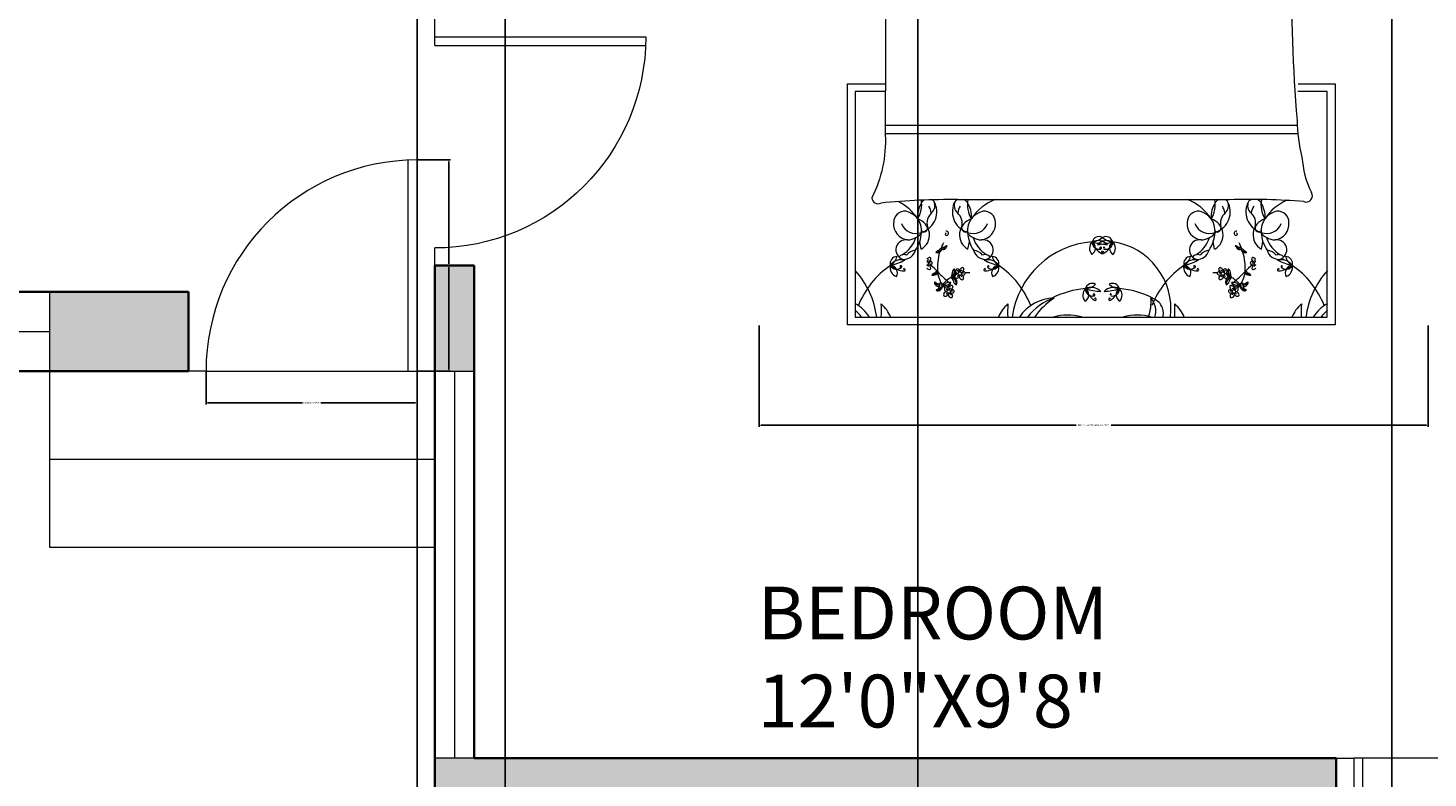
# Model space of a CAD drawing. Units: inches. Extents: x -5 to 366, y -496 to 54.
# Tile 5 of 10: x 121 to 280, y -378 to -293. Entities that reach past the tile are written whole.
import ezdxf

# ---------------------------------------------------------------- set-up
doc = ezdxf.new("R2010")
doc.units = ezdxf.units.IN
doc.header["$MEASUREMENT"] = 0
for name, color, linetype, lineweight in [('A-ANNO-DIMS', 2, 'Continuous', 18), ('A-AREA-IDEN', 7, 'Continuous', 25), ('A-DOOR', 3, 'Continuous', 18), ('A-FLOR-STRS', 7, 'Continuous', 18), ('A-FURN', 8, 'Continuous', 18), ('A-GLAZ', 4, 'Continuous', 18), ('A-WALL', 7, 'Continuous', 35), ('A-WALL-PATT', 252, 'Continuous', 13)]:
    doc.layers.add(name, color=color, linetype=linetype, lineweight=lineweight)
doc.styles.get("Standard").update_dxf_attribs({"font": 'arial.ttf'})
doc.dimstyles.get("Standard").update_dxf_attribs({"dimtxt": 0.18, "dimasz": 0.18, "dimexe": 0.18, "dimexo": 0.0625, "dimgap": 0.09, "dimtad": 0, "dimtih": 1, "dimtoh": 1, "dimdec": 0, "dimzin": 0, "dimdsep": 46, "dimlunit": 3, "dimtxsty": 'Standard', "dimcen": 0.09, "dimadec": 0, "dimazin": 0, "dimtfac": 1, "dimtdec": 0, "dimtofl": 0, "dimtmove": 0, "dimatfit": 3, "dimfxl": 1, "dimtolj": 1, "dimtzin": 0, "dimarcsym": 0})

# ---------------------------------------------------------------- blocks, each defined once
blk = doc.blocks.new('DOOR-SWING-24IN')
for p, q in [((-1, 0), (-1, 24)), ((0, 0), (0, 24))]:
    blk.add_line(p, q)
blk.add_arc((0, 0), 24, 90, 180)
blk = doc.blocks.new('BED-DOUBLE-WITH-NIGHTSTANDS')
for p, q in [((0, 64.67), (76.05, 64.67)), ((15.21, 64.67), (15.21, 43.8)), ((60.84, 63.7), (15.21, 63.7)), ((7.61, 53.37), (7.61, 63.31)), ((68.45, 53.37), (68.45, 63.31)), ((12.58, 58.34), (2.64, 58.34)), ((63.48, 58.34), (73.42, 58.34)), ((15.21, 52.66), (60.84, 52.66)), ((25.78, 50.4), (34.07, 52.66)), ((36.11, 52.66), (31.94, 46.86)), ((20.23, 48.39), (25.78, 50.4)), ((60.64, 49.5), (33.56, 49.12)), ((17.3, 46.24), (20.23, 48.39)), ((60.61, 48.72), (33, 48.33)), ((14.53, 43.01), (17.3, 46.24)), ((31.94, 46.86), (30.24, 42.39)), ((60.57, 46.32), (31.69, 46.21)), ((60.58, 45.54), (31.39, 45.42)), ((15.15, 42.39), (14.53, 43.01)), ((18.23, 42.7), (15.15, 42.39)), ((22.08, 42.39), (18.23, 42.7)), ((25.47, 41.93), (22.08, 42.39)), ((27.47, 41.01), (25.47, 41.93)), ((30.24, 42.39), (29.94, 40.39)), ((29.94, 40.39), (27.47, 41.01)), ((10.04, 27.39), (14.34, 27.39)), ((10.04, 0), (10.04, 27.39)), ((61.27, 27.39), (65.49, 27.39)), ((65.49, 27.39), (65.49, 0)), ((14.34, 26.51), (10.92, 26.51)), ((10.92, 26.51), (10.92, 0.88)), ((64.6, 26.51), (61.25, 26.51)), ((64.6, 0.88), (64.6, 26.51)), ((61.19, 22.65), (14.34, 22.65)), ((61.26, 21.7), (14.34, 21.7)), ((53.47, 14.23), (22.59, 14.23)), ((18.42, 8.59), (18.25, 9.45)), ((23.73, 8.59), (23.9, 9.45)), ((51.79, 8.59), (51.63, 9.45)), ((57.11, 8.59), (57.28, 9.45)), ((10.92, 0.88), (64.6, 0.88)), ((65.49, 0), (10.04, 0))]:
    blk.add_line(p, q)
for points in [[(15.21, 52), (0, 52), (0, 64.67)], [(60.84, 64.67), (60.84, 52), (76.05, 52), (76.05, 64.67)], [(7.61, 58.34), (8.49, 59.87)], [(68.45, 58.34), (67.56, 59.87)], [(7.61, 58.34), (8.49, 56.8)], [(68.45, 58.34), (67.56, 56.8)]]:
    blk.add_lwpolyline(points)
for points in [[(19.58, 62.78, 0.074897), (19.67, 57.81, -0.472817)], [(37.67, 57.53, 0.14099), (37.82, 62.6, 0.235245)], [(40.92, 57.53, -0.14099), (40.77, 62.6, -0.235245)], [(56.48, 62.78, -0.074897), (56.38, 57.81, 0.472817)], [(14.37, 36.04, 0.001242), (14.34, 21.61, -0.127202), (12.81, 14.42)], [(61.17, 23.25, 0.056112), (61.72, 19.07, 0.095341), (62.79, 15.03)]]:
    blk.add_lwpolyline(points, format="xyb")
for centre, radius in [((7.61, 58.34), 3.55), ((68.45, 58.34), 3.55), ((7.61, 58.34), 1.77), ((68.45, 58.34), 1.77), ((22.81, 5.83), 0.194), ((52.72, 5.83), 0.194), ((21.54, 3.79), 0.194), ((53.98, 3.79), 0.194)]:
    blk.add_circle(centre, radius)
for centre, radius, start, end in [((61.5, 786.54), 724.98, 266.68521, 267.14978), ((30, 35.26), 27.58, 82.2196, 99.497), ((35.83, 49.2), 13.55, 81.5249, 103.96), ((41.81, 58.99), 3.76, 63.3437, 106.1026), ((47.45, 49.47), 13.37, 76.3427, 101.1841), ((14.56, 786.54), 724.98, 272.85022, 273.31479), ((29.27, 55.82), 9.8, 155.1316, 191.7583), ((46.79, 55.82), 9.8, 348.2417, 24.8684), ((28.71, 54.99), 9.32, 354.0129, 15.8293), ((49.88, 54.99), 9.32, 164.1707, 185.9871), ((27.66, 70.91), 17.68, 258.0397, 289.2615), ((49.36, 62.92), 9.68, 243.8761, 286.1746), ((22.29, 63.67), 10.19, 255.1039, 281.0369), ((34.82, 67.05), 13.41, 259.8617, 283.6238), ((42.32, 57.67), 4.03, 245.0183, 288.5407), ((53.76, 63.67), 10.19, 258.9631, 284.8961), ((197.18, 43.36), 136.65, 176.1, 180.9282), ((-55.2, 41.12), 69.76, 355.8294, 1.553), ((15.83, 69.94), 28.7, 267.4519, 281.3392), ((22.69, 35.73), 6.19, 66.2616, 101.3392), ((35.22, 69.13), 29.49, 250.1194, 259.3383), ((29.76, 40.33), 0.184, 268.8623, 19.7536), ((238.78, 38.39), 178.26, 179.1145, 184.8735), ((13.51, 14.47), 0.702, 183.98, 297.3412), ((62.21, 14.65), 0.693, 246.5219, 33.8264), ((21.68, -64.93), 79.17, 89.3433, 95.6887), ((16.57, 11.64), 1.28, 84.4856, 181.0538), ((13.22, 8.88), 5.76, 33.6671, 63.2997), ((16.17, 10.69), 2.29, 355.2933, 76.921), ((20.93, 12.3), 2.93, 145.785, 184.7304), ((15.33, 13.67), 3.15, 328.8218, 9.1554), ((19.23, 13.39), 0.916, 120.0293, 142.325), ((17.77, 12.85), 2.42, 289.2822, 29.1751), ((17.4, 12.41), 2.19, 7.436, 29.9149), ((18.84, 13.57), 1.14, 311.5653, 23.8354), ((19.23, 13.39), 0.916, 44.4517, 63.558), ((24.38, 12.85), 2.42, 150.8249, 250.7178), ((23.31, 13.57), 1.14, 156.1646, 228.4347), ((22.92, 13.39), 0.916, 113.229, 135.5483), ((24.75, 12.41), 2.19, 150.0851, 172.564), ((22.92, 13.39), 0.916, 37.675, 66.7144), ((21.22, 12.3), 2.93, 355.2696, 34.215), ((26.82, 13.67), 3.15, 169.7133, 211.1782), ((25.97, 10.69), 2.29, 103.079, 184.7067), ((28.93, 8.88), 5.76, 111.4941, 146.3329), ((25.58, 11.64), 1.28, 358.9462, 95.5144), ((49.95, 11.64), 1.28, 84.4856, 181.0538), ((46.59, 8.88), 5.76, 33.6671, 68.5059), ((49.55, 10.69), 2.29, 355.2933, 76.921), ((54.31, 12.3), 2.93, 145.785, 184.7304), ((48.7, 13.67), 3.15, 328.8218, 10.2867), ((52.61, 13.39), 0.916, 113.2856, 142.325), ((51.15, 12.85), 2.42, 289.2822, 29.1751), ((50.78, 12.41), 2.19, 7.436, 29.9149), ((52.61, 13.39), 0.916, 44.4517, 66.7144), ((52.22, 13.57), 1.14, 311.5653, 23.8354), ((55.8, -59.74), 74, 85.2402, 91.8035), ((57.76, 12.85), 2.42, 150.8249, 250.7178), ((56.68, 13.57), 1.14, 156.1646, 228.4347), ((56.3, 13.39), 0.916, 106.6343, 135.5483), ((58.13, 12.41), 2.19, 150.0851, 172.564), ((56.3, 13.39), 0.916, 37.675, 72.5814), ((54.6, 12.3), 2.93, 355.2696, 34.215), ((60.2, 13.67), 3.15, 169.249, 211.1782), ((59.35, 10.69), 2.29, 103.079, 184.7067), ((62.31, 8.88), 5.76, 113.6453, 146.3329), ((58.96, 11.64), 1.28, 358.9462, 95.5144), ((17.09, 11.46), 1.82, 174.9449, 262.8857), ((17.81, 12.15), 1.76, 201.5819, 291.4221), ((17.47, 10.23), 1.89, 299.9085, 73.1337), ((18.67, 11.02), 0.472, 257.3041, 15.1471), ((20.63, 11.55), 1.56, 131.5653, 195.1471), ((21.52, 11.55), 1.56, 344.8529, 48.4347), ((24.67, 10.23), 1.89, 106.8663, 240.0915), ((23.48, 11.02), 0.472, 164.8529, 282.6959), ((24.34, 12.15), 1.76, 248.5779, 338.4181), ((25.05, 11.46), 1.82, 277.1143, 5.0551), ((50.47, 11.46), 1.82, 174.9449, 262.8857), ((51.19, 12.15), 1.76, 201.5819, 291.4221), ((50.85, 10.23), 1.89, 299.9085, 73.1337), ((52.05, 11.02), 0.472, 257.3041, 15.1471), ((54.01, 11.55), 1.56, 131.5653, 195.1471), ((54.89, 11.55), 1.56, 344.8529, 48.4347), ((58.05, 10.23), 1.89, 106.8663, 240.0915), ((56.86, 11.02), 0.472, 164.8529, 282.6959), ((57.72, 12.15), 1.76, 248.5779, 338.4181), ((58.43, 11.46), 1.82, 277.1143, 5.0551), ((16.68, 8.53), 1.14, 80.264, 250.8688), ((14.41, 11.04), 3.59, 301.2614, 341.7045), ((16.78, 11.86), 2.21, 272.3591, 324.0401), ((14.38, 10.75), 4.08, 326.2883, 356.5076), ((20.93, 12.3), 2.93, 212.7011, 216.3445), ((21.29, 10.31), 0.147, 102.7051, 280.4384), ((21.28, 10.4), 0.238, 280.4384, 100.4136), ((21.22, 12.3), 2.93, 323.6555, 327.2989), ((25.37, 11.86), 2.21, 215.9599, 267.6409), ((27.77, 10.75), 4.08, 183.4924, 213.7117), ((27.73, 11.04), 3.59, 198.2955, 238.7386), ((25.47, 8.53), 1.14, 289.1312, 99.736), ((38.64, 9.21), 0.823, 63.0274, 163.8037), ((37.8, 11.14), 1.7, 271.4585, 315.3727), ((38.49, 8.01), 1.57, 45.5411, 114.3101), ((39.57, 8.01), 1.57, 65.6899, 134.4589), ((39.42, 9.21), 0.823, 16.1963, 116.9726), ((40.26, 11.14), 1.7, 224.6273, 268.5415), ((50.06, 8.53), 1.14, 80.264, 250.8688), ((47.79, 11.04), 3.59, 301.2614, 341.7045), ((50.16, 11.86), 2.21, 272.3591, 324.0401), ((47.76, 10.75), 4.08, 326.2883, 356.5076), ((54.31, 12.3), 2.93, 212.7011, 216.3445), ((54.25, 10.4), 0.238, 79.5864, 259.5616), ((54.23, 10.31), 0.147, 259.5616, 77.2949), ((54.6, 12.3), 2.93, 323.6555, 327.2989), ((58.75, 11.86), 2.21, 215.9599, 267.6409), ((61.15, 10.75), 4.08, 183.4924, 213.7117), ((61.11, 11.04), 3.59, 198.2955, 238.7386), ((58.85, 8.53), 1.14, 289.1312, 99.736), ((16.44, 7.29), 0.7, 63.9755, 143.2681), ((16.4, 8.87), 1.43, 265.969, 344.3045), ((17.94, 6.98), 1.52, 96.1662, 141.5825), ((20.45, 8.04), 0.399, 101.3256, 154.4621), ((19.88, 9.4), 1.2, 280.2588, 300.656), ((20.15, 10.36), 2.14, 268.3264, 277.1302), ((26.56, 6.48), 6.3, 163.5842, 183.8277), ((19.62, 9.39), 1.22, 308.2101, 316.3071), ((20.37, 8.59), 0.365, 278.3432, 4.2869), ((20.17, 8.91), 0.637, 300.656, 332.6341), ((20.64, 8.49), 0.155, 55.7657, 157.4417), ((26.56, 6.48), 6.3, 153.0032, 159.8941), ((20.89, 8.63), 0.155, 84.3784, 186.0543), ((20.74, 9.25), 0.637, 269.1859, 301.164), ((20.93, 8.93), 0.365, 237.5332, 323.4768), ((20.57, 9.97), 1.22, 285.5129, 293.6099), ((21.37, 8.59), 0.399, 87.3579, 140.4944), ((20.45, 9.74), 1.2, 301.164, 321.5612), ((19.47, 9.95), 2.14, 324.6898, 333.4936), ((24.21, 6.98), 1.52, 38.4175, 83.8338), ((25.74, 8.87), 1.43, 195.6955, 274.031), ((25.71, 7.29), 0.7, 36.7319, 116.0245), ((38.62, -0.46), 9.93, 94.4623, 172.255), ((38.66, 8.7), 1.1, 137.7873, 219.1145), ((37.41, 8.74), 0.829, 298.5391, 58.3627), ((39.93, 16.07), 6.95, 252.593, 267.2582), ((38.66, 9.41), 0.812, 177.7585, 283.852), ((40.22, 10.26), 2.51, 198.9159, 238.011), ((38.14, 16.07), 6.95, 272.7418, 287.407), ((38.83, 8.73), 0.107, 283.852, 219.9245), ((38.96, 8.23), 0.123, 238.011, 71.5592), ((38.98, 8.29), 0.0599, 71.5592, 188.0167), ((39.1, 8.23), 0.123, 108.4408, 301.989), ((39.08, 8.29), 0.0599, 351.9833, 108.4408), ((39.22, 8.77), 0.0647, 320.1909, 256.0209), ((37.84, 10.26), 2.51, 301.989, 341.0841), ((39.4, 9.41), 0.812, 256.148, 2.2415), ((40.65, 8.74), 0.829, 121.6373, 241.4609), ((39.4, 8.7), 1.1, 320.8855, 42.2127), ((39.12, 1.83), 7.69, 352.8636, 81.8197), ((49.82, 7.29), 0.7, 63.9755, 143.2681), ((49.78, 8.87), 1.43, 265.969, 344.3045), ((51.32, 6.98), 1.52, 96.1662, 141.5825), ((55.08, 9.74), 1.2, 218.4388, 238.836), ((54.15, 8.59), 0.399, 39.5056, 92.6421), ((56.06, 9.95), 2.14, 206.5064, 215.3102), ((54.6, 8.93), 0.365, 216.5232, 302.4668), ((54.95, 9.97), 1.22, 246.3901, 254.4871), ((54.79, 9.25), 0.637, 238.836, 270.8141), ((48.96, 6.48), 6.3, 20.1059, 26.9968), ((54.64, 8.63), 0.155, 353.9457, 95.6216), ((54.88, 8.49), 0.155, 22.5583, 124.2343), ((55.16, 8.59), 0.365, 175.7131, 261.6568), ((55.36, 8.91), 0.637, 207.3659, 239.344), ((48.96, 6.48), 6.3, 356.1723, 16.4158), ((55.91, 9.39), 1.22, 223.6929, 231.7899), ((55.65, 9.4), 1.2, 239.344, 259.7412), ((55.37, 10.36), 2.14, 262.8698, 271.6736), ((55.07, 8.04), 0.399, 25.5379, 78.6744), ((59.12, 8.87), 1.43, 195.6955, 274.031), ((57.59, 6.98), 1.52, 38.4175, 83.8338), ((59.08, 7.29), 0.7, 36.7319, 116.0245), ((20.52, -1.44), 9.93, 124.3865, 158.5908), ((15.99, 6.52), 1.1, 167.7115, 249.0387), ((15.71, 6.95), 0.823, 92.9516, 193.728), ((14.03, 8.2), 1.7, 301.3827, 345.2969), ((16.18, 5.84), 1.57, 75.4653, 144.2343), ((13.4, 13.54), 6.95, 282.5173, 297.1824), ((14.89, 5.93), 0.829, 328.4633, 88.2869), ((16.56, 8.65), 2.51, 228.8402, 267.9352), ((15.63, 7.13), 0.812, 207.6827, 313.7762), ((16.12, 6.62), 0.107, 313.7762, 249.7183), ((16.46, 6.32), 0.0599, 101.4834, 217.9409), ((16.48, 6.26), 0.123, 267.9352, 101.4834), ((19.32, 7.28), 0.323, 101.5637, 142.6358), ((19.06, 6.98), 0.194, 273.2768, 86.7232), ((19.32, 6.63), 0.32, 217.7621, 259.0403), ((19.28, 7.17), 0.185, 91.1081, 181.8675), ((19.66, 7.05), 0.588, 203.4276, 227.6104), ((19.48, 6.8), 0.4, 80.3487, 133.6538), ((19.41, 7.13), 0.317, 229.7889, 317.6792), ((19.06, 7.54), 0.466, 288.7263, 352.5032), ((19.05, 6.46), 0.45, 355.053, 68.3618), ((19.4, 6.38), 0.634, 83.0852, 105.7171), ((19.38, 7.52), 0.15, 345.2356, 144.9248), ((19.35, 6.43), 0.149, 232.4737, 355.053), ((15.01, 1.12), 7.22, 43.1541, 52.0459), ((19.52, 7.03), 0.167, 317.6792, 80.3487), ((21.33, 6.12), 0.883, 304.5369, 16.3699), ((22.55, 5.87), 0.625, 127.3105, 187.9252), ((21.7, 5.94), 0.641, 355.0106, 41.658), ((23.08, 6.13), 0.323, 101.5637, 176.365), ((23.14, 6.36), 0.15, 345.2356, 144.9248), ((25.67, 6.26), 0.123, 78.5166, 272.0648), ((25.96, 5.84), 1.57, 35.7657, 104.5347), ((28.74, 13.54), 6.95, 242.8176, 257.4827), ((25.58, 8.65), 2.51, 272.0648, 311.1598), ((25.68, 6.32), 0.0599, 322.0591, 78.5166), ((26.52, 7.13), 0.812, 226.2238, 332.3173), ((26.04, 6.66), 0.0647, 290.2667, 226.2271), ((27.26, 5.93), 0.829, 91.7131, 211.5367), ((26.44, 6.95), 0.823, 346.272, 87.0484), ((28.12, 8.2), 1.7, 194.7031, 238.6173), ((26.16, 6.52), 1.1, 290.9613, 12.2885), ((21.63, -1.44), 9.93, 21.4092, 55.6135), ((53.9, -1.44), 9.93, 124.3865, 158.5908), ((49.36, 6.52), 1.1, 167.7115, 249.0387), ((49.09, 6.95), 0.823, 92.9516, 193.728), ((47.41, 8.2), 1.7, 301.3827, 345.2969), ((49.56, 5.84), 1.57, 75.4653, 144.2343), ((46.78, 13.54), 6.95, 282.5173, 297.1824), ((49.01, 7.13), 0.812, 207.6827, 313.7762), ((49.94, 8.65), 2.51, 228.8402, 267.9352), ((48.26, 5.93), 0.829, 328.4633, 88.2869), ((49.5, 6.62), 0.107, 313.7762, 249.7183), ((49.84, 6.32), 0.0599, 101.4834, 217.9409), ((49.86, 6.26), 0.123, 267.9352, 101.4834), ((52.39, 6.36), 0.15, 35.0752, 194.7644), ((52.45, 6.13), 0.323, 3.635, 78.4363), ((53.83, 5.94), 0.641, 138.342, 184.9894), ((54.2, 6.12), 0.883, 163.6301, 235.4631), ((52.97, 5.87), 0.625, 352.0748, 52.6895), ((60.52, 1.12), 7.22, 127.9541, 136.8459), ((56.01, 7.03), 0.167, 99.6513, 222.3208), ((56.12, 7.13), 0.317, 222.3208, 310.2111), ((56.05, 6.8), 0.4, 46.3462, 99.6513), ((56.15, 7.52), 0.15, 35.0752, 194.7644), ((56.46, 7.54), 0.466, 187.4968, 251.2737), ((56.48, 6.46), 0.45, 111.6382, 184.947), ((56.18, 6.43), 0.149, 184.947, 307.5263), ((56.12, 6.38), 0.634, 74.2829, 96.9148), ((56.25, 7.17), 0.185, 358.1325, 88.8919), ((55.86, 7.05), 0.588, 312.3896, 336.5724), ((56.2, 7.28), 0.323, 37.3642, 78.4363), ((56.21, 6.63), 0.32, 280.9597, 322.2379), ((56.47, 6.98), 0.194, 93.2768, 266.7232), ((59.05, 6.26), 0.123, 78.5166, 272.0648), ((59.34, 5.84), 1.57, 35.7657, 104.5347), ((62.12, 13.54), 6.95, 242.8176, 257.4827), ((58.96, 8.65), 2.51, 272.0648, 311.1598), ((59.06, 6.32), 0.0599, 322.0591, 78.5166), ((59.9, 7.13), 0.812, 226.2238, 332.3173), ((59.42, 6.66), 0.0647, 290.2667, 226.2271), ((60.64, 5.93), 0.829, 91.7131, 211.5367), ((61.5, 8.2), 1.7, 194.7031, 238.6173), ((59.82, 6.95), 0.823, 346.272, 87.0484), ((59.54, 6.52), 1.1, 290.9613, 12.2885), ((55.01, -1.44), 9.93, 21.4092, 55.6135), ((3.53, -0.46), 9.93, 7.745, 41.8856), ((20, 5.48), 0.399, 101.3256, 154.4621), ((19.42, 6.84), 1.2, 280.2588, 300.656), ((19.7, 7.8), 2.14, 268.3264, 277.1302), ((19.17, 6.83), 1.22, 308.2101, 316.3071), ((20.13, 4.78), 0.216, 146.8636, 236.9021), ((23.18, 9.55), 5.66, 235.1882, 238.8844), ((20.5, 5.1), 0.585, 199.4799, 267.6828), ((19.91, 6.03), 0.365, 278.3432, 4.2869), ((19.71, 6.35), 0.637, 300.656, 332.6341), ((20.19, 5.93), 0.155, 55.7657, 157.4417), ((23.43, 6.32), 3.16, 184.756, 209.2041), ((27.97, 13.04), 10.39, 222.2412, 232.1744), ((20.65, 4.61), 0.169, 311.8703, 134.2646), ((21.14, 5.38), 0.883, 247.2305, 319.0635), ((23.75, 2.13), 3.79, 120.544, 139.818), ((21.59, 4.21), 0.625, 70.0041, 130.6188), ((21.19, 4.97), 0.641, 297.7043, 344.3516), ((21.8, 5.92), 0.537, 272.8499, 356.1226), ((21.42, 5.72), 0.52, 321.7607, 7.9252), ((21.53, 4.97), 0.52, 8.7227, 54.8872), ((21.56, 4.55), 0.883, 0.278, 72.111), ((21.95, 4.88), 0.537, 20.5253, 88.5375), ((22.66, 5.14), 0.625, 188.7227, 249.3375), ((22.4, 5.47), 0.192, 148.0499, 225.6268), ((23.75, 2.13), 3.79, 113.0501, 113.8477), ((22.76, 5.25), 0.611, 104.7558, 148.0499), ((22.42, 5.69), 0.382, 247.4086, 351.4386), ((22.6, 6.1), 0.264, 126.1046, 271.4281), ((22.57, 6.17), 0.19, 353.7526, 131.7054), ((21.86, 4.83), 0.641, 334.9899, 21.6373), ((22.52, 5.67), 0.128, 262.906, 7.132), ((22.39, 5.95), 0.267, 0.0645, 61.1507), ((22.45, 6.18), 0.305, 311.8413, 355.7877), ((23.07, 5.47), 0.32, 151.2196, 259.0403), ((23.04, 6.02), 0.185, 91.1081, 181.8675), ((23.42, 5.9), 0.588, 203.4276, 227.6104), ((23.23, 5.64), 0.4, 80.3487, 133.6538), ((23.16, 5.98), 0.317, 229.7889, 317.6792), ((22.82, 6.39), 0.466, 288.7263, 352.5032), ((22.8, 5.3), 0.45, 355.053, 68.3618), ((23.16, 5.23), 0.634, 83.0852, 105.7171), ((23.1, 5.28), 0.149, 232.4737, 355.053), ((23.27, 5.87), 0.167, 317.6792, 80.3487), ((23.75, 2.13), 3.79, 87.1071, 94.7585), ((51.78, 2.13), 3.79, 85.2415, 92.8929), ((52.25, 5.87), 0.167, 99.6513, 222.3208), ((52.37, 5.98), 0.317, 222.3208, 310.2111), ((52.29, 5.64), 0.4, 46.3462, 99.6513), ((52.71, 6.39), 0.466, 187.4968, 251.2737), ((52.72, 5.3), 0.45, 111.6382, 184.947), ((52.42, 5.28), 0.149, 184.947, 307.5263), ((52.37, 5.23), 0.634, 74.2829, 96.9148), ((52.49, 6.02), 0.185, 358.1325, 88.8919), ((52.11, 5.9), 0.588, 312.3896, 336.5724), ((52.45, 5.47), 0.32, 280.9597, 28.7804), ((53.11, 5.69), 0.382, 188.5614, 292.5914), ((52.96, 6.17), 0.19, 48.2946, 186.2474), ((53.07, 6.18), 0.305, 184.2123, 228.1587), ((53.14, 5.95), 0.267, 118.8493, 179.9355), ((53, 5.67), 0.128, 172.868, 277.094), ((52.93, 6.1), 0.264, 268.5719, 53.8954), ((52.77, 5.25), 0.611, 31.9501, 75.2442), ((53.67, 4.83), 0.641, 158.3627, 205.0101), ((53.57, 4.88), 0.537, 91.4625, 159.4747), ((53.97, 4.55), 0.883, 107.889, 179.722), ((52.87, 5.14), 0.625, 290.6625, 351.2773), ((53.73, 5.92), 0.537, 183.8774, 267.1501), ((51.78, 2.13), 3.79, 66.1523, 66.9499), ((53.12, 5.47), 0.192, 314.3732, 31.9501), ((54, 4.97), 0.52, 125.1128, 171.2773), ((54.11, 5.72), 0.52, 172.0748, 218.2393), ((51.78, 2.13), 3.79, 40.182, 59.456), ((53.93, 4.21), 0.625, 49.3812, 109.9959), ((54.39, 5.38), 0.883, 220.9365, 292.7695), ((54.34, 4.97), 0.641, 195.6484, 242.2957), ((47.55, 13.04), 10.39, 307.8256, 317.7588), ((54.88, 4.61), 0.169, 45.7354, 228.1297), ((52.1, 6.32), 3.16, 330.7959, 355.244), ((55.02, 5.1), 0.585, 272.3172, 340.5201), ((55.33, 5.93), 0.155, 22.5583, 124.2343), ((55.61, 6.03), 0.365, 175.7131, 261.6568), ((55.81, 6.35), 0.637, 207.3659, 239.344), ((52.34, 9.55), 5.66, 301.1156, 304.8118), ((56.36, 6.83), 1.22, 223.6929, 231.7899), ((56.1, 6.84), 1.2, 239.344, 259.7412), ((55.39, 4.78), 0.216, 303.0979, 33.1364), ((55.82, 7.8), 2.14, 262.8698, 271.6736), ((55.53, 5.48), 0.399, 25.5379, 78.6744), ((72, -0.46), 9.93, 138.1144, 172.255), ((20.44, 4.87), 0.504, 212.8155, 277.3992), ((20.15, 4.54), 0.585, 266.9701, 338.2913), ((17.06, 8.72), 5.66, 302.6784, 306.3746), ((20.29, 4.07), 0.216, 214.3538, 304.3923), ((20.37, 4.89), 0.224, 238.8844, 314.2646), ((20.33, 4.39), 0.504, 280.3057, 17.1958), ((20.28, 4.34), 0.224, 306.3746, 21.7548), ((20.65, 4.49), 0.169, 19.3605, 201.7548), ((23.82, 3.07), 3.37, 153.7819, 158.2913), ((20.85, 5.08), 0.52, 264.4544, 310.6188), ((23.43, 6.32), 3.16, 214.0033, 222.4917), ((21.23, 4.87), 0.537, 218.3208, 298.8162), ((21.14, 3.43), 0.192, 148.0499, 225.6268), ((21.49, 3.21), 0.611, 104.7558, 148.0499), ((21.15, 3.64), 0.382, 247.4086, 351.4386), ((21.33, 4.06), 0.264, 126.1046, 271.4281), ((21.3, 4.13), 0.19, 353.7526, 131.7054), ((21.26, 3.63), 0.128, 262.906, 7.132), ((21.12, 3.91), 0.267, 0.0645, 61.1507), ((21.18, 4.13), 0.305, 311.8413, 355.7877), ((21.81, 4.09), 0.323, 101.5637, 176.365), ((21.81, 3.43), 0.32, 151.2196, 259.0403), ((21.77, 3.98), 0.185, 91.1081, 181.8675), ((22.15, 3.86), 0.588, 203.4276, 227.6104), ((21.97, 3.6), 0.4, 80.3487, 133.6538), ((21.89, 3.93), 0.317, 229.7889, 317.6792), ((21.55, 4.35), 0.466, 288.7263, 352.5032), ((21.54, 3.26), 0.45, 355.053, 68.3618), ((21.89, 3.19), 0.634, 83.0852, 105.7171), ((21.87, 4.32), 0.15, 345.2356, 144.9248), ((21.84, 3.24), 0.149, 232.4737, 355.053), ((22, 3.83), 0.167, 317.6792, 80.3487), ((37.86, -5.78), 9.93, 94.4623, 117.4146), ((37.9, 3.38), 1.1, 137.7873, 219.1145), ((36.65, 3.42), 0.829, 298.5391, 58.3627), ((37.88, 3.89), 0.823, 63.0274, 163.8037), ((37.04, 5.82), 1.7, 271.4585, 315.3727), ((37.73, 2.69), 1.57, 45.5411, 114.3101), ((39.46, 4.94), 2.51, 198.9159, 238.011), ((39.17, 10.75), 6.95, 252.593, 267.2582), ((37.9, 4.09), 0.812, 177.7585, 283.852), ((38.07, 3.41), 0.107, 283.852, 219.9245), ((40.33, 2.69), 1.57, 65.6899, 134.4589), ((38.9, 10.75), 6.95, 272.7418, 287.407), ((40.18, 3.89), 0.823, 16.1963, 116.9726), ((41.02, 5.82), 1.7, 224.6273, 268.5415), ((39.98, 3.45), 0.0647, 320.1909, 256.0209), ((38.6, 4.94), 2.51, 301.989, 341.0841), ((40.16, 4.09), 0.812, 256.148, 2.2415), ((41.41, 3.42), 0.829, 121.6373, 241.4609), ((40.16, 3.38), 1.1, 320.8855, 42.2127), ((40.2, -5.78), 9.93, 62.5854, 85.5377), ((53.52, 3.83), 0.167, 99.6513, 222.3208), ((53.63, 3.93), 0.317, 222.3208, 310.2111), ((53.56, 3.6), 0.4, 46.3462, 99.6513), ((53.66, 4.32), 0.15, 35.0752, 194.7644), ((53.97, 4.35), 0.466, 187.4968, 251.2737), ((53.99, 3.26), 0.45, 111.6382, 184.947), ((53.69, 3.24), 0.149, 184.947, 307.5263), ((53.64, 3.19), 0.634, 74.2829, 96.9148), ((53.76, 3.98), 0.185, 358.1325, 88.8919), ((53.37, 3.86), 0.588, 312.3896, 336.5724), ((53.72, 4.09), 0.323, 3.635, 78.4363), ((53.72, 3.43), 0.32, 280.9597, 28.7804), ((54.38, 3.64), 0.382, 188.5614, 292.5914), ((54.3, 4.87), 0.537, 241.1838, 321.6792), ((54.23, 4.13), 0.19, 48.2946, 186.2474), ((54.34, 4.13), 0.305, 184.2123, 228.1587), ((54.4, 3.91), 0.267, 118.8493, 179.9355), ((54.27, 3.63), 0.128, 172.868, 277.094), ((54.2, 4.06), 0.264, 268.5719, 53.8954), ((54.03, 3.21), 0.611, 31.9501, 75.2442), ((54.68, 5.08), 0.52, 229.3812, 275.5456), ((52.1, 6.32), 3.16, 317.5083, 325.9967), ((54.39, 3.43), 0.192, 314.3732, 31.9501), ((55.2, 4.39), 0.504, 162.8042, 259.6943), ((54.88, 4.49), 0.169, 338.2452, 160.6395), ((51.7, 3.07), 3.37, 21.7087, 26.2181), ((55.38, 4.54), 0.585, 201.7087, 273.0299), ((55.15, 4.89), 0.224, 225.7354, 301.1156), ((55.09, 4.87), 0.504, 262.6008, 327.1845), ((55.24, 4.34), 0.224, 158.2452, 233.6254), ((58.47, 8.72), 5.66, 233.6254, 237.3216), ((55.23, 4.07), 0.216, 235.6077, 325.6462), ((8.51, -1.79), 4.84, 33.4617, 60.1116), ((6.77, -2.69), 6.03, 36.3036, 46.4814), ((11.22, -0.67), 4.04, 22.5547, 48.9546), ((0.16, 1.5), 13.74, 357.4081, 3.6519), ((30.93, -0.67), 4.04, 131.0454, 157.4453), ((41.99, 1.5), 13.74, 176.3481, 182.5919), ((33.64, -1.79), 4.84, 91.272, 146.5383), ((35.38, -2.69), 6.03, 107.8504, 143.6964), ((38.55, -4.39), 8.97, 124.0123, 144.053), ((38.2, 2.91), 0.123, 238.011, 71.5592), ((38.22, 2.97), 0.0599, 71.5592, 188.0167), ((39.86, 2.91), 0.123, 108.4408, 301.989), ((39.84, 2.97), 0.0599, 351.9833, 108.4408), ((40.11, 2.54), 4.45, 338.117, 6.6195), ((44.19, 1.3), 1.78, 346.3898, 79.0739), ((42.85, 1.54), 2.25, 342.8609, 41.9049), ((33.54, 1.5), 13.74, 357.4081, 3.6519), ((44.6, -0.67), 4.04, 22.5547, 48.9546), ((64.31, -0.67), 4.04, 131.0454, 157.4453), ((75.37, 1.5), 13.74, 176.3481, 182.5919), ((67.02, -1.79), 4.84, 119.8884, 146.5383), ((68.76, -2.69), 6.03, 133.5186, 143.6964), ((35.08, -4.34), 5.46, 73.5431, 107.0202), ((37.25, -7.16), 8.08, 94.3787, 95.6357), ((41.5, -12.69), 14.43, 109.7217, 109.9028), ((42.98, -4.34), 5.46, 72.9798, 106.4569), ((40.82, -7.16), 8.08, 84.3643, 85.6213), ((36.56, -12.69), 14.43, 70.0972, 70.2783)]:
    blk.add_arc(centre, radius, start, end)
blk = doc.blocks.new('*D11')
at = {"layer": 'A-ANNO-DIMS', "color": 0, "lineweight": -2, "transparency": 16777216}
for p, q in [((141.43, -332.04), (141.43, -335.76)), ((165.43, -332.04), (165.43, -335.76)), ((141.61, -335.58), (152.39, -335.58)), ((165.25, -335.58), (154.48, -335.58))]:
    blk.add_line(p, q, dxfattribs=at)
at = {"layer": 'A-ANNO-DIMS', "color": 0, "transparency": 16777216}
for points in [[(141.61, -335.55), (141.61, -335.61), (141.43, -335.58)], [(165.25, -335.55), (165.25, -335.61), (165.43, -335.58)]]:
    blk.add_solid(points, dxfattribs=at)
at = {"layer": 'Defpoints', "color": 0, "transparency": 16777216}
for p in [(141.43, -331.98), (165.43, -331.98), (165.43, -335.58)]:
    blk.add_point(p, dxfattribs=at)
at = {"layer": 'A-ANNO-DIMS', "color": 0, "transparency": 16777216, "insert": (153.43, -335.58), "char_height": 0.18, "attachment_point": 5}
blk.add_mtext('\\A1;DOOR 2\'-0" TYP.', dxfattribs=at)
blk = doc.blocks.new('*D12')
at = {"layer": 'A-ANNO-DIMS', "color": 0, "lineweight": -2, "transparency": 16777216}
for p, q in [((165.5, -307.98), (169.21, -307.98)), ((169.03, -308.16), (169.03, -319.8)), ((169.03, -331.8), (169.03, -320.16)), ((165.5, -331.98), (169.21, -331.98))]:
    blk.add_line(p, q, dxfattribs=at)
at = {"layer": 'A-ANNO-DIMS', "color": 0, "transparency": 16777216}
for points in [[(169, -308.16), (169.06, -308.16), (169.03, -307.98)], [(169, -331.8), (169.06, -331.8), (169.03, -331.98)]]:
    blk.add_solid(points, dxfattribs=at)
at = {"layer": 'Defpoints', "color": 0, "transparency": 16777216}
for p in [(165.43, -307.98), (169.03, -307.98), (165.43, -331.98)]:
    blk.add_point(p, dxfattribs=at)
at = {"layer": 'A-ANNO-DIMS', "color": 0, "transparency": 16777216, "insert": (169.03, -319.98), "char_height": 0.18, "attachment_point": 5}
blk.add_mtext('\\A1;2\'-0" TYP.', dxfattribs=at)
blk = doc.blocks.new('*D15')
at = {"layer": 'A-ANNO-DIMS', "color": 0, "lineweight": -2, "transparency": 16777216}
for p, q in [((204.33, -326.78), (204.33, -338.31)), ((280.38, -326.78), (280.38, -338.31)), ((204.51, -338.13), (240.37, -338.13)), ((280.2, -338.13), (244.34, -338.13))]:
    blk.add_line(p, q, dxfattribs=at)
at = {"layer": 'A-ANNO-DIMS', "color": 0, "transparency": 16777216}
for points in [[(204.51, -338.1), (204.51, -338.16), (204.33, -338.13)], [(280.2, -338.1), (280.2, -338.16), (280.38, -338.13)]]:
    blk.add_solid(points, dxfattribs=at)
at = {"layer": 'Defpoints', "color": 0, "transparency": 16777216}
for p in [(204.33, -326.72), (280.38, -326.72), (280.38, -338.13)]:
    blk.add_point(p, dxfattribs=at)
at = {"layer": 'A-ANNO-DIMS', "color": 0, "transparency": 16777216, "insert": (242.35, -338.13), "char_height": 0.18, "attachment_point": 5}
blk.add_mtext('\\A1;BED & NIGHTSTANDS 6\'-4" TYP.', dxfattribs=at)
blk = doc.blocks.new('*D29')
at = {"layer": 'A-ANNO-DIMS', "color": 0, "lineweight": -2, "transparency": 16777216}
for p, q in [((165.43, -380.42), (165.43, 53.15)), ((165.61, 52.97), (170.03, 52.97)), ((175.25, 52.97), (170.83, 52.97)), ((175.43, -380.42), (175.43, 53.15))]:
    blk.add_line(p, q, dxfattribs=at)
at = {"layer": 'A-ANNO-DIMS', "color": 0, "transparency": 16777216}
for points in [[(165.61, 53), (165.61, 52.94), (165.43, 52.97)], [(175.25, 53), (175.25, 52.94), (175.43, 52.97)]]:
    blk.add_solid(points, dxfattribs=at)
at = {"layer": 'Defpoints', "color": 0, "transparency": 16777216}
for p in [(175.43, 52.97), (165.43, -380.48), (175.43, -380.48)]:
    blk.add_point(p, dxfattribs=at)
at = {"layer": 'A-ANNO-DIMS', "color": 0, "transparency": 16777216, "insert": (170.43, 52.97), "char_height": 0.18, "attachment_point": 5}
blk.add_mtext('\\A1;0\'-10"', dxfattribs=at)
blk = doc.blocks.new('*D32')
at = {"layer": 'A-ANNO-DIMS', "color": 0, "lineweight": -2, "transparency": 16777216}
for p, q in [((222.37, -254.15), (222.37, -495.61)), ((276.25, -254.15), (276.25, -495.61)), ((222.55, -495.43), (248.98, -495.43)), ((276.07, -495.43), (249.64, -495.43))]:
    blk.add_line(p, q, dxfattribs=at)
at = {"layer": 'A-ANNO-DIMS', "color": 0, "transparency": 16777216}
for points in [[(222.55, -495.4), (222.55, -495.46), (222.37, -495.43)], [(276.07, -495.4), (276.07, -495.46), (276.25, -495.43)]]:
    blk.add_solid(points, dxfattribs=at)
at = {"layer": 'Defpoints', "color": 0, "transparency": 16777216}
for p in [(222.37, -254.09), (276.25, -254.09), (276.25, -495.43)]:
    blk.add_point(p, dxfattribs=at)
at = {"layer": 'A-ANNO-DIMS', "color": 0, "transparency": 16777216, "insert": (249.31, -495.43), "char_height": 0.18, "attachment_point": 5}
blk.add_mtext('\\A1;4\'-6"', dxfattribs=at)

msp = doc.modelspace()

# ---------------------------------------------------------------- hatches: boundary and pattern name
at = {"layer": 'A-WALL-PATT'}
h = msp.add_hatch(color=256, dxfattribs=at)
h.dxf.hatch_style = 1
h.paths.add_polyline_path([(187.93, -13.98), (183.43, -13.98), (163.43, -13.98), (163.43, -18.48), (183.43, -18.48), (183.43, -74.48), (185.68, -74.48), (187.93, -74.48)])
h.paths.add_polyline_path([(284.93, -102.48), (215.93, -102.48), (215.93, -104.73), (215.93, -106.98), (280.43, -106.98), (284.93, -106.98)])
h.paths.add_polyline_path([(284.93, -133.23), (280.43, -133.23), (280.43, -154.98), (220.43, -154.98), (220.43, -134.98), (215.93, -134.98), (215.93, -159.48), (284.93, -159.48)])
h.paths.add_polyline_path([(139.43, -322.98), (123.64, -322.98), (123.64, -331.98), (139.43, -331.98)])
h.paths.add_polyline_path([(171.93, -319.98), (167.43, -319.98), (167.43, -331.98), (171.93, -331.98)])
h.paths.add_polyline_path([(269.93, -375.98), (171.93, -375.98), (167.43, -375.98), (167.43, -380.48), (171.93, -380.48), (265.43, -380.48), (265.43, -452.48), (171.93, -452.48), (167.43, -452.48), (167.43, -456.98), (281.67, -456.98), (281.67, -452.48), (269.93, -452.48), (269.93, -380.48)])

# ---------------------------------------------------------------- linework, layer by layer
at = {"layer": 'A-DOOR'}
for p, q in [((167.43, -294.98), (167.43, -291.98)), ((167.43, -319.98), (167.43, -317.98)), ((141.43, -331.98), (139.43, -331.98)), ((141.43, -331.98), (165.43, -331.98)), ((167.43, -331.98), (165.43, -331.98)), ((269.93, -375.98), (271.93, -375.98)), ((295.93, -375.98), (271.93, -375.98))]:
    msp.add_line(p, q, dxfattribs=at)
at = {"layer": 'A-FLOR-STRS'}
for p, q in [((123.64, -331.98), (123.64, -341.98)), ((123.64, -341.98), (123.64, -351.98)), ((123.64, -341.98), (167.43, -341.98)), ((123.64, -351.98), (167.43, -351.98))]:
    msp.add_line(p, q, dxfattribs=at)
at = {"layer": 'A-GLAZ'}
for p, q in [((123.64, -322.98), (123.64, -331.98)), ((30.93, -327.48), (123.64, -327.48)), ((167.43, -331.98), (171.93, -331.98)), ((169.68, -331.98), (169.68, -375.98)), ((171.93, -375.98), (167.43, -375.98))]:
    msp.add_line(p, q, dxfattribs=at)
at = {"layer": 'A-WALL'}
for p, q in [((171.93, -319.98), (167.43, -319.98)), ((167.43, -319.98), (167.43, -380.48)), ((171.93, -319.98), (171.93, -375.98)), ((30.93, -322.98), (139.43, -322.98)), ((139.43, -331.98), (139.43, -322.98)), ((26.43, -331.98), (139.43, -331.98)), ((171.93, -375.98), (269.93, -375.98)), ((269.93, -380.48), (269.93, -375.98))]:
    msp.add_line(p, q, dxfattribs=at)

# ---------------------------------------------------------------- block references
at = {"layer": 'A-DOOR', "extrusion": (0, 0, -1), "zscale": -1, "rotation": 90.00000000000007}
msp.add_blockref('DOOR-SWING-24IN', (-167.43, -293.98), dxfattribs=at)
at = {"layer": 'A-DOOR'}
msp.add_blockref('DOOR-SWING-24IN', (165.43, -331.98), dxfattribs=at)
at = {"layer": 'A-DOOR', "rotation": 180}
msp.add_blockref('DOOR-SWING-24IN', (271.93, -375.98), dxfattribs=at)
at = {"layer": 'A-FURN'}
msp.add_blockref('BED-DOUBLE-WITH-NIGHTSTANDS', (204.33, -326.72), dxfattribs=at)

# ---------------------------------------------------------------- texts
at = {"layer": 'A-AREA-IDEN', "insert": (204.16, -356.48), "char_height": 6, "attachment_point": 1}
msp.add_mtext('BEDROOM\\P12\'0"X9\'8"', dxfattribs=at)

# ---------------------------------------------------------------- dimensions: what is measured, and where the dimension line sits
at = {"layer": 'A-ANNO-DIMS'}
for base, p1, p2, picture, middle in [((175.43, 52.97), (165.43, -380.48), (175.43, -380.48), '*D29', (170.43, 52.97)), ((276.25, -495.43), (222.37, -254.09), (276.25, -254.09), '*D32', (249.31, -495.43))]:
    dim = msp.add_linear_dim(base=base, p1=p1, p2=p2, dimstyle='Standard', override={"dimdec": 1, "dimlfac": 1, "dimrnd": 0, "dimzin": 1, "dimdsep": 46, "dimlunit": 4, "dimfrac": 2}, dxfattribs=at)
    dim.commit()
    dim.dimension.update_dxf_attribs({"geometry": picture, "text_midpoint": middle})
dim = msp.add_linear_dim(base=(169.03, -307.98), p1=(165.43, -331.98), p2=(165.43, -307.98), angle=90, text='<> TYP.', dimstyle='Standard', override={"dimdec": 1, "dimlfac": 1, "dimrnd": 0, "dimzin": 1, "dimdsep": 46, "dimlunit": 4, "dimfrac": 2}, dxfattribs=at)
dim.commit()
dim.dimension.update_dxf_attribs({"geometry": '*D12', "text_midpoint": (169.03, -319.98)})
for base, p1, p2, text, picture, middle in [((280.38, -338.1282), (204.3279, -326.7204), (280.38, -326.7204), 'BED & NIGHTSTANDS <> TYP.', '*D15', (242.3539, -338.1282)), ((165.43, -335.58), (141.43, -331.98), (165.43, -331.98), 'DOOR <> TYP.', '*D11', (153.43, -335.58))]:
    dim = msp.add_linear_dim(base=base, p1=p1, p2=p2, text=text, dimstyle='Standard', override={"dimdec": 1, "dimlfac": 1, "dimrnd": 0, "dimzin": 1, "dimdsep": 46, "dimlunit": 4, "dimfrac": 2}, dxfattribs=at)
    dim.commit()
    dim.dimension.update_dxf_attribs({"geometry": picture, "text_midpoint": middle})

doc.saveas('drawing.dxf')
